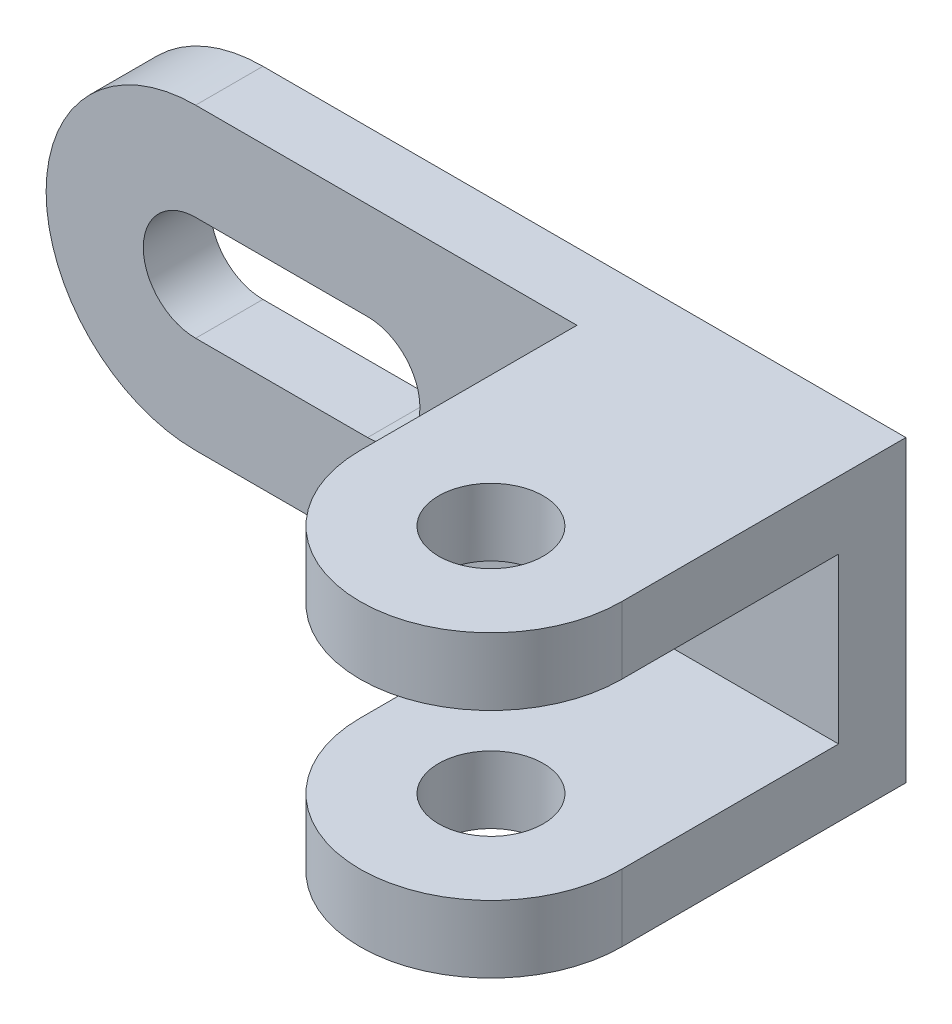
ISO-10303-21;
HEADER;
FILE_DESCRIPTION(('STEP AP214'),'2;1');
FILE_NAME('part.step','',(''),(''),'','','');
FILE_SCHEMA(('AUTOMOTIVE_DESIGN { 1 0 10303 214 1 1 1 1 }'));
ENDSEC;
DATA;
#1=APPLICATION_CONTEXT('core data for automotive mechanical design processes');
#2=APPLICATION_PROTOCOL_DEFINITION('international standard','automotive_design',2000,#1);
#3=PRODUCT_CONTEXT('',#1,'mechanical');
#4=PRODUCT('Part','Part','',(#3));
#5=PRODUCT_RELATED_PRODUCT_CATEGORY('part','',(#4));
#6=PRODUCT_DEFINITION_FORMATION('','',#4);
#7=PRODUCT_DEFINITION_CONTEXT('part definition',#1,'design');
#8=PRODUCT_DEFINITION('design','',#6,#7);
#9=PRODUCT_DEFINITION_SHAPE('','',#8);
#10=(LENGTH_UNIT() NAMED_UNIT(*) SI_UNIT(.MILLI.,.METRE.));
#11=(NAMED_UNIT(*) PLANE_ANGLE_UNIT() SI_UNIT($,.RADIAN.));
#12=(NAMED_UNIT(*) SI_UNIT($,.STERADIAN.) SOLID_ANGLE_UNIT());
#13=UNCERTAINTY_MEASURE_WITH_UNIT(LENGTH_MEASURE(1.E-05),#10,'distance_accuracy_value','');
#14=(GEOMETRIC_REPRESENTATION_CONTEXT(3) GLOBAL_UNCERTAINTY_ASSIGNED_CONTEXT((#13)) GLOBAL_UNIT_ASSIGNED_CONTEXT((#10,
#11,#12)) REPRESENTATION_CONTEXT('',''));
#15=CARTESIAN_POINT('',(0.,0.,0.));
#16=DIRECTION('',(0.,0.,1.));
#17=DIRECTION('',(1.,0.,0.));
#18=AXIS2_PLACEMENT_3D('',#15,#16,#17);
#19=CARTESIAN_POINT('',(-86.,-20.,9.));
#20=DIRECTION('',(0.,0.,-1.));
#21=DIRECTION('',(-1.,0.,0.));
#22=AXIS2_PLACEMENT_3D('',#19,#20,#21);
#23=PLANE('',#22);
#24=DIRECTION('',(-1.,0.,0.));
#25=VECTOR('',#24,1.);
#26=CARTESIAN_POINT('',(-86.,-27.,9.));
#27=LINE('',#26,#25);
#28=CARTESIAN_POINT('',(-63.,-27.,9.));
#29=VERTEX_POINT('',#28);
#30=CARTESIAN_POINT('',(-86.,-27.,9.));
#31=VERTEX_POINT('',#30);
#32=EDGE_CURVE('E223',#29,#31,#27,.T.);
#33=ORIENTED_EDGE('',*,*,#32,.T.);
#34=CARTESIAN_POINT('',(-86.,-20.,9.));
#35=DIRECTION('',(0.,0.,-1.));
#36=DIRECTION('',(-1.,0.,0.));
#37=AXIS2_PLACEMENT_3D('',#34,#35,#36);
#38=CIRCLE('',#37,7.);
#39=CARTESIAN_POINT('',(-86.,-13.,9.));
#40=VERTEX_POINT('',#39);
#41=EDGE_CURVE('E226',#31,#40,#38,.T.);
#42=ORIENTED_EDGE('',*,*,#41,.T.);
#43=DIRECTION('',(1.,0.,0.));
#44=VECTOR('',#43,1.);
#45=CARTESIAN_POINT('',(-86.,-13.,9.));
#46=LINE('',#45,#44);
#47=CARTESIAN_POINT('',(-63.,-13.,9.));
#48=VERTEX_POINT('',#47);
#49=EDGE_CURVE('E214',#40,#48,#46,.T.);
#50=ORIENTED_EDGE('',*,*,#49,.T.);
#51=CARTESIAN_POINT('',(-63.,-20.,9.));
#52=DIRECTION('',(0.,0.,-1.));
#53=DIRECTION('',(-1.,0.,0.));
#54=AXIS2_PLACEMENT_3D('',#51,#52,#53);
#55=CIRCLE('',#54,7.);
#56=EDGE_CURVE('E224',#48,#29,#55,.T.);
#57=ORIENTED_EDGE('',*,*,#56,.T.);
#58=EDGE_LOOP('',(#33,#42,#50,#57));
#59=FACE_BOUND('',#58,.T.);
#60=DIRECTION('',(-1.,0.,0.));
#61=VECTOR('',#60,1.);
#62=CARTESIAN_POINT('',(-35.,-9.,8.99999999999989));
#63=LINE('',#62,#61);
#64=CARTESIAN_POINT('',(0.,-9.,9.));
#65=VERTEX_POINT('',#64);
#66=CARTESIAN_POINT('',(-35.,-9.,9.));
#67=VERTEX_POINT('',#66);
#68=EDGE_CURVE('E54',#65,#67,#63,.T.);
#69=ORIENTED_EDGE('',*,*,#68,.T.);
#70=DIRECTION('',(0.,1.,0.));
#71=VECTOR('',#70,1.);
#72=CARTESIAN_POINT('',(-35.,-9.,8.99999999999989));
#73=LINE('',#72,#71);
#74=CARTESIAN_POINT('',(-35.,0.,8.99999999999989));
#75=VERTEX_POINT('',#74);
#76=EDGE_CURVE('E154',#67,#75,#73,.T.);
#77=ORIENTED_EDGE('',*,*,#76,.T.);
#78=DIRECTION('',(-1.,0.,0.));
#79=VECTOR('',#78,1.);
#80=CARTESIAN_POINT('',(0.,0.,9.));
#81=LINE('',#80,#79);
#82=CARTESIAN_POINT('',(-86.,0.,9.));
#83=VERTEX_POINT('',#82);
#84=EDGE_CURVE('E231',#75,#83,#81,.T.);
#85=ORIENTED_EDGE('',*,*,#84,.T.);
#86=CARTESIAN_POINT('',(-86.,-20.,9.));
#87=DIRECTION('',(0.,0.,1.));
#88=DIRECTION('',(-1.,0.,0.));
#89=AXIS2_PLACEMENT_3D('',#86,#87,#88);
#90=CIRCLE('',#89,20.);
#91=CARTESIAN_POINT('',(-86.,-40.,9.));
#92=VERTEX_POINT('',#91);
#93=EDGE_CURVE('E236',#83,#92,#90,.T.);
#94=ORIENTED_EDGE('',*,*,#93,.T.);
#95=DIRECTION('',(1.,0.,0.));
#96=VECTOR('',#95,1.);
#97=CARTESIAN_POINT('',(0.,-40.,9.));
#98=LINE('',#97,#96);
#99=CARTESIAN_POINT('',(-35.,-40.,8.99999999999989));
#100=VERTEX_POINT('',#99);
#101=EDGE_CURVE('E238',#92,#100,#98,.T.);
#102=ORIENTED_EDGE('',*,*,#101,.T.);
#103=DIRECTION('',(0.,-1.,0.));
#104=VECTOR('',#103,1.);
#105=CARTESIAN_POINT('',(-35.,-31.,8.99999999999989));
#106=LINE('',#105,#104);
#107=CARTESIAN_POINT('',(-35.,-31.,8.99999999999989));
#108=VERTEX_POINT('',#107);
#109=EDGE_CURVE('E200',#108,#100,#106,.T.);
#110=ORIENTED_EDGE('',*,*,#109,.F.);
#111=DIRECTION('',(1.,0.,0.));
#112=VECTOR('',#111,1.);
#113=CARTESIAN_POINT('',(-35.,-31.,8.99999999999989));
#114=LINE('',#113,#112);
#115=CARTESIAN_POINT('',(0.,-31.,9.));
#116=VERTEX_POINT('',#115);
#117=EDGE_CURVE('E182',#108,#116,#114,.T.);
#118=ORIENTED_EDGE('',*,*,#117,.T.);
#119=DIRECTION('',(0.,1.,0.));
#120=VECTOR('',#119,1.);
#121=CARTESIAN_POINT('',(0.,0.,9.));
#122=LINE('',#121,#120);
#123=EDGE_CURVE('E58',#116,#65,#122,.T.);
#124=ORIENTED_EDGE('',*,*,#123,.T.);
#125=EDGE_LOOP('',(#69,#77,#85,#94,#102,#110,#118,#124));
#126=FACE_BOUND('',#125,.T.);
#127=ADVANCED_FACE('F39',(#59,#126),#23,.F.);
#128=CARTESIAN_POINT('',(0.,0.,9.));
#129=DIRECTION('',(-1.,0.,0.));
#130=DIRECTION('',(0.,0.,1.));
#131=AXIS2_PLACEMENT_3D('',#128,#129,#130);
#132=PLANE('',#131);
#133=DIRECTION('',(0.,1.,0.));
#134=VECTOR('',#133,1.);
#135=CARTESIAN_POINT('',(0.,0.,0.));
#136=LINE('',#135,#134);
#137=CARTESIAN_POINT('',(0.,-40.,0.));
#138=VERTEX_POINT('',#137);
#139=CARTESIAN_POINT('',(0.,0.,0.));
#140=VERTEX_POINT('',#139);
#141=EDGE_CURVE('E233',#138,#140,#136,.T.);
#142=ORIENTED_EDGE('',*,*,#141,.T.);
#143=DIRECTION('',(0.,0.,-1.));
#144=VECTOR('',#143,1.);
#145=CARTESIAN_POINT('',(0.,0.,9.));
#146=LINE('',#145,#144);
#147=CARTESIAN_POINT('',(0.,0.,38.));
#148=VERTEX_POINT('',#147);
#149=EDGE_CURVE('E11',#148,#140,#146,.T.);
#150=ORIENTED_EDGE('',*,*,#149,.F.);
#151=DIRECTION('',(0.,1.,0.));
#152=VECTOR('',#151,1.);
#153=CARTESIAN_POINT('',(0.,-9.,38.));
#154=LINE('',#153,#152);
#155=CARTESIAN_POINT('',(0.,-9.,38.));
#156=VERTEX_POINT('',#155);
#157=EDGE_CURVE('E153',#156,#148,#154,.T.);
#158=ORIENTED_EDGE('',*,*,#157,.F.);
#159=DIRECTION('',(0.,0.,-1.));
#160=VECTOR('',#159,1.);
#161=CARTESIAN_POINT('',(0.,-9.,9.));
#162=LINE('',#161,#160);
#163=EDGE_CURVE('E163',#156,#65,#162,.T.);
#164=ORIENTED_EDGE('',*,*,#163,.T.);
#165=ORIENTED_EDGE('',*,*,#123,.F.);
#166=DIRECTION('',(0.,0.,1.));
#167=VECTOR('',#166,1.);
#168=CARTESIAN_POINT('',(0.,-31.,9.));
#169=LINE('',#168,#167);
#170=CARTESIAN_POINT('',(0.,-31.,38.));
#171=VERTEX_POINT('',#170);
#172=EDGE_CURVE('E184',#116,#171,#169,.T.);
#173=ORIENTED_EDGE('',*,*,#172,.T.);
#174=DIRECTION('',(0.,-1.,0.));
#175=VECTOR('',#174,1.);
#176=CARTESIAN_POINT('',(0.,-31.,38.));
#177=LINE('',#176,#175);
#178=CARTESIAN_POINT('',(0.,-40.,38.));
#179=VERTEX_POINT('',#178);
#180=EDGE_CURVE('E194',#171,#179,#177,.T.);
#181=ORIENTED_EDGE('',*,*,#180,.T.);
#182=DIRECTION('',(0.,0.,-1.));
#183=VECTOR('',#182,1.);
#184=CARTESIAN_POINT('',(0.,-40.,9.));
#185=LINE('',#184,#183);
#186=EDGE_CURVE('E241',#179,#138,#185,.T.);
#187=ORIENTED_EDGE('',*,*,#186,.T.);
#188=EDGE_LOOP('',(#142,#150,#158,#164,#165,#173,#181,#187));
#189=FACE_BOUND('',#188,.T.);
#190=ADVANCED_FACE('F41',(#189),#132,.F.);
#191=CARTESIAN_POINT('',(0.,0.,9.));
#192=DIRECTION('',(0.,-1.,0.));
#193=DIRECTION('',(0.,0.,-1.));
#194=AXIS2_PLACEMENT_3D('',#191,#192,#193);
#195=PLANE('',#194);
#196=CARTESIAN_POINT('',(-17.5,0.,38.));
#197=DIRECTION('',(0.,1.,0.));
#198=DIRECTION('',(0.,0.,1.));
#199=AXIS2_PLACEMENT_3D('',#196,#197,#198);
#200=CIRCLE('',#199,7.);
#201=CARTESIAN_POINT('',(-17.5,0.,45.));
#202=VERTEX_POINT('',#201);
#203=EDGE_CURVE('E315',#202,#202,#200,.T.);
#204=ORIENTED_EDGE('',*,*,#203,.F.);
#205=EDGE_LOOP('',(#204));
#206=FACE_BOUND('',#205,.T.);
#207=DIRECTION('',(-1.,0.,0.));
#208=VECTOR('',#207,1.);
#209=CARTESIAN_POINT('',(0.,0.,0.));
#210=LINE('',#209,#208);
#211=CARTESIAN_POINT('',(-86.,0.,0.));
#212=VERTEX_POINT('',#211);
#213=EDGE_CURVE('E242',#140,#212,#210,.T.);
#214=ORIENTED_EDGE('',*,*,#213,.T.);
#215=DIRECTION('',(0.,0.,-1.));
#216=VECTOR('',#215,1.);
#217=CARTESIAN_POINT('',(-86.,0.,9.));
#218=LINE('',#217,#216);
#219=EDGE_CURVE('E48',#83,#212,#218,.T.);
#220=ORIENTED_EDGE('',*,*,#219,.F.);
#221=ORIENTED_EDGE('',*,*,#84,.F.);
#222=DIRECTION('',(0.,0.,1.));
#223=VECTOR('',#222,1.);
#224=CARTESIAN_POINT('',(-35.,0.,38.));
#225=LINE('',#224,#223);
#226=CARTESIAN_POINT('',(-35.,0.,38.));
#227=VERTEX_POINT('',#226);
#228=EDGE_CURVE('E169',#75,#227,#225,.T.);
#229=ORIENTED_EDGE('',*,*,#228,.T.);
#230=CARTESIAN_POINT('',(-17.5,0.,38.));
#231=DIRECTION('',(0.,1.,0.));
#232=DIRECTION('',(0.,0.,-1.));
#233=AXIS2_PLACEMENT_3D('',#230,#231,#232);
#234=CIRCLE('',#233,17.5);
#235=EDGE_CURVE('E149',#227,#148,#234,.T.);
#236=ORIENTED_EDGE('',*,*,#235,.T.);
#237=ORIENTED_EDGE('',*,*,#149,.T.);
#238=EDGE_LOOP('',(#214,#220,#221,#229,#236,#237));
#239=FACE_BOUND('',#238,.T.);
#240=ADVANCED_FACE('F280',(#206,#239),#195,.F.);
#241=CARTESIAN_POINT('',(-86.,-20.,9.));
#242=DIRECTION('',(0.,0.,-1.));
#243=DIRECTION('',(-1.,0.,0.));
#244=AXIS2_PLACEMENT_3D('',#241,#242,#243);
#245=CYLINDRICAL_SURFACE('',#244,20.);
#246=CARTESIAN_POINT('',(-86.,-20.,0.));
#247=DIRECTION('',(0.,0.,1.));
#248=DIRECTION('',(-1.,0.,0.));
#249=AXIS2_PLACEMENT_3D('',#246,#247,#248);
#250=CIRCLE('',#249,20.);
#251=CARTESIAN_POINT('',(-86.,-40.,0.));
#252=VERTEX_POINT('',#251);
#253=EDGE_CURVE('E246',#212,#252,#250,.T.);
#254=ORIENTED_EDGE('',*,*,#253,.T.);
#255=DIRECTION('',(0.,0.,-1.));
#256=VECTOR('',#255,1.);
#257=CARTESIAN_POINT('',(-86.,-40.,9.));
#258=LINE('',#257,#256);
#259=EDGE_CURVE('E252',#92,#252,#258,.T.);
#260=ORIENTED_EDGE('',*,*,#259,.F.);
#261=ORIENTED_EDGE('',*,*,#93,.F.);
#262=ORIENTED_EDGE('',*,*,#219,.T.);
#263=EDGE_LOOP('',(#254,#260,#261,#262));
#264=FACE_BOUND('',#263,.T.);
#265=ADVANCED_FACE('F256',(#264),#245,.T.);
#266=CARTESIAN_POINT('',(0.,-40.,9.));
#267=DIRECTION('',(0.,1.,0.));
#268=DIRECTION('',(-1.,0.,0.));
#269=AXIS2_PLACEMENT_3D('',#266,#267,#268);
#270=PLANE('',#269);
#271=CARTESIAN_POINT('',(-17.5,-40.,38.));
#272=DIRECTION('',(0.,1.,0.));
#273=DIRECTION('',(-1.,0.,0.));
#274=AXIS2_PLACEMENT_3D('',#271,#272,#273);
#275=CIRCLE('',#274,7.);
#276=CARTESIAN_POINT('',(-24.5,-40.,38.));
#277=VERTEX_POINT('',#276);
#278=EDGE_CURVE('E171',#277,#277,#275,.T.);
#279=ORIENTED_EDGE('',*,*,#278,.T.);
#280=EDGE_LOOP('',(#279));
#281=FACE_BOUND('',#280,.T.);
#282=DIRECTION('',(1.,0.,0.));
#283=VECTOR('',#282,1.);
#284=CARTESIAN_POINT('',(0.,-40.,0.));
#285=LINE('',#284,#283);
#286=EDGE_CURVE('E234',#252,#138,#285,.T.);
#287=ORIENTED_EDGE('',*,*,#286,.T.);
#288=ORIENTED_EDGE('',*,*,#186,.F.);
#289=CARTESIAN_POINT('',(-17.5,-40.,38.));
#290=DIRECTION('',(0.,-1.,0.));
#291=DIRECTION('',(1.,0.,0.));
#292=AXIS2_PLACEMENT_3D('',#289,#290,#291);
#293=CIRCLE('',#292,17.5);
#294=CARTESIAN_POINT('',(-35.,-40.,38.));
#295=VERTEX_POINT('',#294);
#296=EDGE_CURVE('E173',#179,#295,#293,.T.);
#297=ORIENTED_EDGE('',*,*,#296,.T.);
#298=DIRECTION('',(0.,0.,-1.));
#299=VECTOR('',#298,1.);
#300=CARTESIAN_POINT('',(-35.,-40.,38.));
#301=LINE('',#300,#299);
#302=EDGE_CURVE('E179',#295,#100,#301,.T.);
#303=ORIENTED_EDGE('',*,*,#302,.T.);
#304=ORIENTED_EDGE('',*,*,#101,.F.);
#305=ORIENTED_EDGE('',*,*,#259,.T.);
#306=EDGE_LOOP('',(#287,#288,#297,#303,#304,#305));
#307=FACE_BOUND('',#306,.T.);
#308=ADVANCED_FACE('F269',(#281,#307),#270,.F.);
#309=CARTESIAN_POINT('',(-86.,-20.,0.));
#310=DIRECTION('',(0.,0.,-1.));
#311=DIRECTION('',(-1.,0.,0.));
#312=AXIS2_PLACEMENT_3D('',#309,#310,#311);
#313=PLANE('',#312);
#314=CARTESIAN_POINT('',(-86.,-20.,0.));
#315=DIRECTION('',(0.,0.,-1.));
#316=DIRECTION('',(0.,1.,0.));
#317=AXIS2_PLACEMENT_3D('',#314,#315,#316);
#318=CIRCLE('',#317,7.);
#319=CARTESIAN_POINT('',(-86.,-27.,0.));
#320=VERTEX_POINT('',#319);
#321=CARTESIAN_POINT('',(-86.,-13.,0.));
#322=VERTEX_POINT('',#321);
#323=EDGE_CURVE('E197',#320,#322,#318,.T.);
#324=ORIENTED_EDGE('',*,*,#323,.F.);
#325=DIRECTION('',(-1.,0.,0.));
#326=VECTOR('',#325,1.);
#327=CARTESIAN_POINT('',(-86.,-27.,0.));
#328=LINE('',#327,#326);
#329=CARTESIAN_POINT('',(-63.,-27.,0.));
#330=VERTEX_POINT('',#329);
#331=EDGE_CURVE('E210',#330,#320,#328,.T.);
#332=ORIENTED_EDGE('',*,*,#331,.F.);
#333=CARTESIAN_POINT('',(-63.,-20.,0.));
#334=DIRECTION('',(0.,0.,-1.));
#335=DIRECTION('',(0.,1.,0.));
#336=AXIS2_PLACEMENT_3D('',#333,#334,#335);
#337=CIRCLE('',#336,7.);
#338=CARTESIAN_POINT('',(-63.,-13.,0.));
#339=VERTEX_POINT('',#338);
#340=EDGE_CURVE('E201',#339,#330,#337,.T.);
#341=ORIENTED_EDGE('',*,*,#340,.F.);
#342=DIRECTION('',(1.,0.,0.));
#343=VECTOR('',#342,1.);
#344=CARTESIAN_POINT('',(-86.,-13.,0.));
#345=LINE('',#344,#343);
#346=EDGE_CURVE('E202',#322,#339,#345,.T.);
#347=ORIENTED_EDGE('',*,*,#346,.F.);
#348=EDGE_LOOP('',(#324,#332,#341,#347));
#349=FACE_BOUND('',#348,.T.);
#350=ORIENTED_EDGE('',*,*,#141,.F.);
#351=ORIENTED_EDGE('',*,*,#286,.F.);
#352=ORIENTED_EDGE('',*,*,#253,.F.);
#353=ORIENTED_EDGE('',*,*,#213,.F.);
#354=EDGE_LOOP('',(#350,#351,#352,#353));
#355=FACE_BOUND('',#354,.T.);
#356=ADVANCED_FACE('F261',(#349,#355),#313,.T.);
#357=CARTESIAN_POINT('',(-86.,-20.,28.));
#358=DIRECTION('',(0.,0.,-1.));
#359=DIRECTION('',(0.,1.,0.));
#360=AXIS2_PLACEMENT_3D('',#357,#358,#359);
#361=CYLINDRICAL_SURFACE('',#360,7.);
#362=DIRECTION('',(0.,0.,-1.));
#363=VECTOR('',#362,1.);
#364=CARTESIAN_POINT('',(-86.,-27.,28.));
#365=LINE('',#364,#363);
#366=EDGE_CURVE('E212',#31,#320,#365,.T.);
#367=ORIENTED_EDGE('',*,*,#366,.T.);
#368=ORIENTED_EDGE('',*,*,#323,.T.);
#369=DIRECTION('',(0.,0.,-1.));
#370=VECTOR('',#369,1.);
#371=CARTESIAN_POINT('',(-86.,-13.,28.));
#372=LINE('',#371,#370);
#373=EDGE_CURVE('E208',#40,#322,#372,.T.);
#374=ORIENTED_EDGE('',*,*,#373,.F.);
#375=ORIENTED_EDGE('',*,*,#41,.F.);
#376=EDGE_LOOP('',(#367,#368,#374,#375));
#377=FACE_BOUND('',#376,.T.);
#378=ADVANCED_FACE('F298',(#377),#361,.F.);
#379=CARTESIAN_POINT('',(-86.,-27.,28.));
#380=DIRECTION('',(0.,-1.,0.));
#381=DIRECTION('',(0.,0.,-1.));
#382=AXIS2_PLACEMENT_3D('',#379,#380,#381);
#383=PLANE('',#382);
#384=DIRECTION('',(0.,0.,-1.));
#385=VECTOR('',#384,1.);
#386=CARTESIAN_POINT('',(-63.,-27.,28.));
#387=LINE('',#386,#385);
#388=EDGE_CURVE('E211',#29,#330,#387,.T.);
#389=ORIENTED_EDGE('',*,*,#388,.T.);
#390=ORIENTED_EDGE('',*,*,#331,.T.);
#391=ORIENTED_EDGE('',*,*,#366,.F.);
#392=ORIENTED_EDGE('',*,*,#32,.F.);
#393=EDGE_LOOP('',(#389,#390,#391,#392));
#394=FACE_BOUND('',#393,.T.);
#395=ADVANCED_FACE('F339',(#394),#383,.F.);
#396=CARTESIAN_POINT('',(-63.,-20.,28.));
#397=DIRECTION('',(0.,0.,-1.));
#398=DIRECTION('',(0.,1.,0.));
#399=AXIS2_PLACEMENT_3D('',#396,#397,#398);
#400=CYLINDRICAL_SURFACE('',#399,7.);
#401=DIRECTION('',(0.,0.,-1.));
#402=VECTOR('',#401,1.);
#403=CARTESIAN_POINT('',(-63.,-13.,28.));
#404=LINE('',#403,#402);
#405=EDGE_CURVE('E217',#48,#339,#404,.T.);
#406=ORIENTED_EDGE('',*,*,#405,.T.);
#407=ORIENTED_EDGE('',*,*,#340,.T.);
#408=ORIENTED_EDGE('',*,*,#388,.F.);
#409=ORIENTED_EDGE('',*,*,#56,.F.);
#410=EDGE_LOOP('',(#406,#407,#408,#409));
#411=FACE_BOUND('',#410,.T.);
#412=ADVANCED_FACE('F345',(#411),#400,.F.);
#413=CARTESIAN_POINT('',(-86.,-13.,28.));
#414=DIRECTION('',(0.,1.,0.));
#415=DIRECTION('',(0.,0.,1.));
#416=AXIS2_PLACEMENT_3D('',#413,#414,#415);
#417=PLANE('',#416);
#418=ORIENTED_EDGE('',*,*,#373,.T.);
#419=ORIENTED_EDGE('',*,*,#346,.T.);
#420=ORIENTED_EDGE('',*,*,#405,.F.);
#421=ORIENTED_EDGE('',*,*,#49,.F.);
#422=EDGE_LOOP('',(#418,#419,#420,#421));
#423=FACE_BOUND('',#422,.T.);
#424=ADVANCED_FACE('F336',(#423),#417,.F.);
#425=CARTESIAN_POINT('',(-17.5,-31.,38.));
#426=DIRECTION('',(0.,-1.,0.));
#427=DIRECTION('',(1.,0.,0.));
#428=AXIS2_PLACEMENT_3D('',#425,#426,#427);
#429=CYLINDRICAL_SURFACE('',#428,17.5);
#430=ORIENTED_EDGE('',*,*,#296,.F.);
#431=ORIENTED_EDGE('',*,*,#180,.F.);
#432=CARTESIAN_POINT('',(-17.5,-31.,38.));
#433=DIRECTION('',(0.,-1.,0.));
#434=DIRECTION('',(1.,0.,0.));
#435=AXIS2_PLACEMENT_3D('',#432,#433,#434);
#436=CIRCLE('',#435,17.5);
#437=CARTESIAN_POINT('',(-35.,-31.,38.));
#438=VERTEX_POINT('',#437);
#439=EDGE_CURVE('E176',#171,#438,#436,.T.);
#440=ORIENTED_EDGE('',*,*,#439,.T.);
#441=DIRECTION('',(0.,-1.,0.));
#442=VECTOR('',#441,1.);
#443=CARTESIAN_POINT('',(-35.,-31.,38.));
#444=LINE('',#443,#442);
#445=EDGE_CURVE('E189',#438,#295,#444,.T.);
#446=ORIENTED_EDGE('',*,*,#445,.T.);
#447=EDGE_LOOP('',(#430,#431,#440,#446));
#448=FACE_BOUND('',#447,.T.);
#449=ADVANCED_FACE('F271',(#448),#429,.T.);
#450=CARTESIAN_POINT('',(-35.,-31.,38.));
#451=DIRECTION('',(-1.,0.,0.));
#452=DIRECTION('',(0.,0.,1.));
#453=AXIS2_PLACEMENT_3D('',#450,#451,#452);
#454=PLANE('',#453);
#455=ORIENTED_EDGE('',*,*,#302,.F.);
#456=ORIENTED_EDGE('',*,*,#445,.F.);
#457=DIRECTION('',(0.,0.,-1.));
#458=VECTOR('',#457,1.);
#459=CARTESIAN_POINT('',(-35.,-31.,38.));
#460=LINE('',#459,#458);
#461=EDGE_CURVE('E177',#438,#108,#460,.T.);
#462=ORIENTED_EDGE('',*,*,#461,.T.);
#463=ORIENTED_EDGE('',*,*,#109,.T.);
#464=EDGE_LOOP('',(#455,#456,#462,#463));
#465=FACE_BOUND('',#464,.T.);
#466=ADVANCED_FACE('F335',(#465),#454,.T.);
#467=CARTESIAN_POINT('',(-17.5,-31.,38.));
#468=DIRECTION('',(0.,-1.,0.));
#469=DIRECTION('',(1.,0.,0.));
#470=AXIS2_PLACEMENT_3D('',#467,#468,#469);
#471=PLANE('',#470);
#472=CARTESIAN_POINT('',(-17.5,-31.,38.));
#473=DIRECTION('',(0.,-1.,0.));
#474=DIRECTION('',(1.,0.,0.));
#475=AXIS2_PLACEMENT_3D('',#472,#473,#474);
#476=CIRCLE('',#475,7.);
#477=CARTESIAN_POINT('',(-10.5,-31.,38.));
#478=VERTEX_POINT('',#477);
#479=EDGE_CURVE('E308',#478,#478,#476,.T.);
#480=ORIENTED_EDGE('',*,*,#479,.T.);
#481=EDGE_LOOP('',(#480));
#482=FACE_BOUND('',#481,.T.);
#483=ORIENTED_EDGE('',*,*,#439,.F.);
#484=ORIENTED_EDGE('',*,*,#172,.F.);
#485=ORIENTED_EDGE('',*,*,#117,.F.);
#486=ORIENTED_EDGE('',*,*,#461,.F.);
#487=EDGE_LOOP('',(#483,#484,#485,#486));
#488=FACE_BOUND('',#487,.T.);
#489=ADVANCED_FACE('F326',(#482,#488),#471,.F.);
#490=CARTESIAN_POINT('',(-17.5,-9.,38.));
#491=DIRECTION('',(0.,1.,0.));
#492=DIRECTION('',(0.,0.,1.));
#493=AXIS2_PLACEMENT_3D('',#490,#491,#492);
#494=CYLINDRICAL_SURFACE('',#493,17.5);
#495=ORIENTED_EDGE('',*,*,#235,.F.);
#496=DIRECTION('',(0.,1.,0.));
#497=VECTOR('',#496,1.);
#498=CARTESIAN_POINT('',(-35.,-9.,38.));
#499=LINE('',#498,#497);
#500=CARTESIAN_POINT('',(-35.,-9.,38.));
#501=VERTEX_POINT('',#500);
#502=EDGE_CURVE('E142',#501,#227,#499,.T.);
#503=ORIENTED_EDGE('',*,*,#502,.F.);
#504=CARTESIAN_POINT('',(-17.5,-9.,38.));
#505=DIRECTION('',(0.,1.,0.));
#506=DIRECTION('',(0.,0.,-1.));
#507=AXIS2_PLACEMENT_3D('',#504,#505,#506);
#508=CIRCLE('',#507,17.5);
#509=EDGE_CURVE('E143',#501,#156,#508,.T.);
#510=ORIENTED_EDGE('',*,*,#509,.T.);
#511=ORIENTED_EDGE('',*,*,#157,.T.);
#512=EDGE_LOOP('',(#495,#503,#510,#511));
#513=FACE_BOUND('',#512,.T.);
#514=ADVANCED_FACE('F141',(#513),#494,.T.);
#515=CARTESIAN_POINT('',(-35.,-9.,38.));
#516=DIRECTION('',(-1.,0.,0.));
#517=DIRECTION('',(0.,0.,1.));
#518=AXIS2_PLACEMENT_3D('',#515,#516,#517);
#519=PLANE('',#518);
#520=ORIENTED_EDGE('',*,*,#228,.F.);
#521=ORIENTED_EDGE('',*,*,#76,.F.);
#522=DIRECTION('',(0.,0.,1.));
#523=VECTOR('',#522,1.);
#524=CARTESIAN_POINT('',(-35.,-9.,38.));
#525=LINE('',#524,#523);
#526=EDGE_CURVE('E156',#67,#501,#525,.T.);
#527=ORIENTED_EDGE('',*,*,#526,.T.);
#528=ORIENTED_EDGE('',*,*,#502,.T.);
#529=EDGE_LOOP('',(#520,#521,#527,#528));
#530=FACE_BOUND('',#529,.T.);
#531=ADVANCED_FACE('F161',(#530),#519,.T.);
#532=CARTESIAN_POINT('',(-17.5,-9.,38.));
#533=DIRECTION('',(0.,-1.,0.));
#534=DIRECTION('',(0.,0.,-1.));
#535=AXIS2_PLACEMENT_3D('',#532,#533,#534);
#536=PLANE('',#535);
#537=CARTESIAN_POINT('',(-17.5,-8.99999999999999,38.));
#538=DIRECTION('',(0.,-1.,0.));
#539=DIRECTION('',(0.,0.,-1.));
#540=AXIS2_PLACEMENT_3D('',#537,#538,#539);
#541=CIRCLE('',#540,7.);
#542=CARTESIAN_POINT('',(-17.5,-8.99999999999999,31.));
#543=VERTEX_POINT('',#542);
#544=EDGE_CURVE('E43',#543,#543,#541,.T.);
#545=ORIENTED_EDGE('',*,*,#544,.F.);
#546=EDGE_LOOP('',(#545));
#547=FACE_BOUND('',#546,.T.);
#548=ORIENTED_EDGE('',*,*,#68,.F.);
#549=ORIENTED_EDGE('',*,*,#163,.F.);
#550=ORIENTED_EDGE('',*,*,#509,.F.);
#551=ORIENTED_EDGE('',*,*,#526,.F.);
#552=EDGE_LOOP('',(#548,#549,#550,#551));
#553=FACE_BOUND('',#552,.T.);
#554=ADVANCED_FACE('F160',(#547,#553),#536,.T.);
#555=CARTESIAN_POINT('',(-17.5,-80.,38.));
#556=DIRECTION('',(0.,1.,0.));
#557=DIRECTION('',(0.,0.,1.));
#558=AXIS2_PLACEMENT_3D('',#555,#556,#557);
#559=CYLINDRICAL_SURFACE('',#558,7.);
#560=ORIENTED_EDGE('',*,*,#544,.T.);
#561=EDGE_LOOP('',(#560));
#562=FACE_BOUND('',#561,.T.);
#563=ORIENTED_EDGE('',*,*,#203,.T.);
#564=EDGE_LOOP('',(#563));
#565=FACE_BOUND('',#564,.T.);
#566=ADVANCED_FACE('F319',(#562,#565),#559,.F.);
#567=ORIENTED_EDGE('',*,*,#479,.F.);
#568=EDGE_LOOP('',(#567));
#569=FACE_BOUND('',#568,.T.);
#570=ORIENTED_EDGE('',*,*,#278,.F.);
#571=EDGE_LOOP('',(#570));
#572=FACE_BOUND('',#571,.T.);
#573=ADVANCED_FACE('F323',(#569,#572),#559,.F.);
#574=CLOSED_SHELL('',(#127,#190,#240,#265,#308,#356,#378,#395,#412,#424,#449,#466,#489,#514,
#531,#554,#566,#573));
#575=MANIFOLD_SOLID_BREP('B2',#574);
#576=ADVANCED_BREP_SHAPE_REPRESENTATION('',(#18,#575),#14);
#577=SHAPE_DEFINITION_REPRESENTATION(#9,#576);
ENDSEC;
END-ISO-10303-21;
